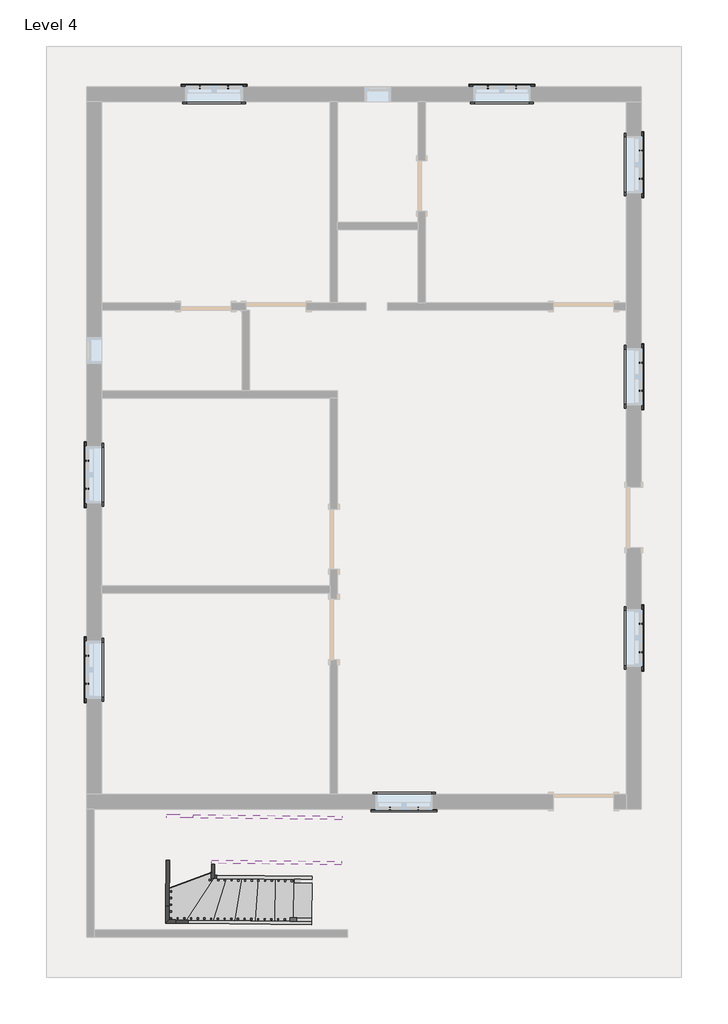
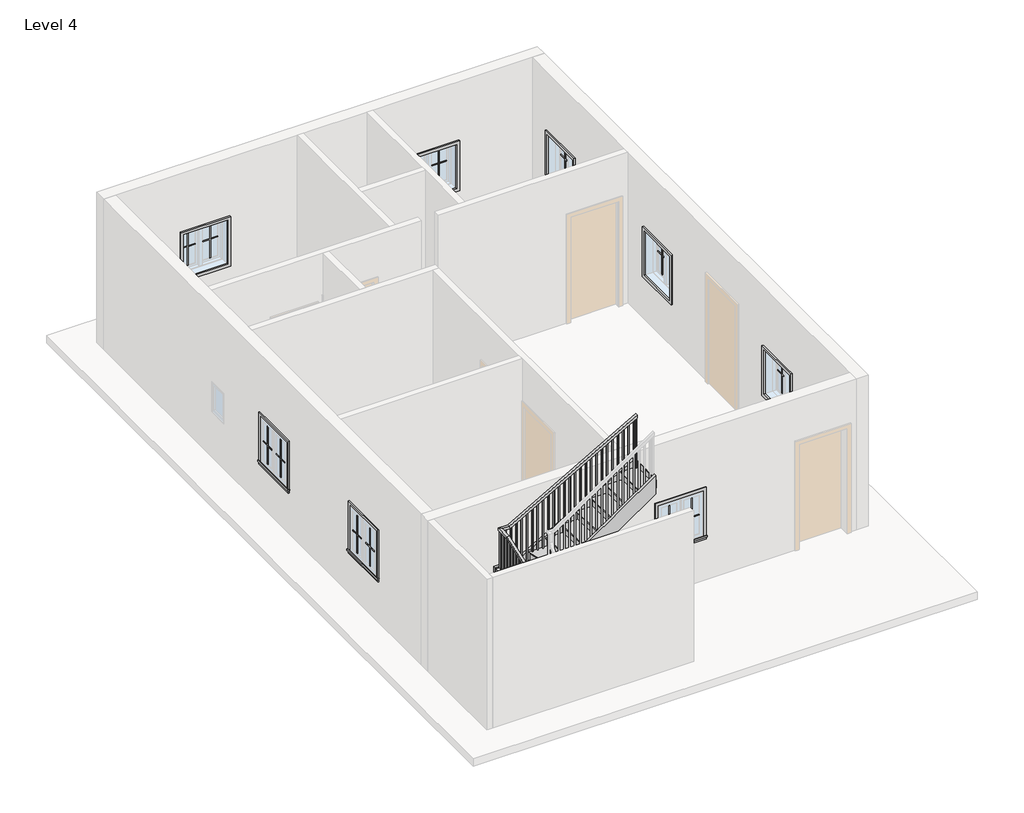
# One storey, part 2 of 2: 32 proxies, 9 members, 1 railing, 1 stair flight.
"""IFC4 building model written with IfcOpenShell, lengths in millimetres."""

from ifc_helpers import new_model, si_unit, frame, origin, place, context, project, spatial, polyline, outline, extrude, faceted_brep, transform, mapped, element, save
from components import muntin_pattern_2x2_muntin_pattern_2x2_b3fe6957, muntin_pattern_2x2_muntin_pattern_2x2_3e0ecaf2, trim_window_exterior_flat_with_sill_41619996, trim_window_interior_flat_picture_frame_51c85655, stair_flight_64b704a5

model = new_model("IFC4")

# Units and contexts
model_context = context("Model", 3, world=origin())
ifc_project = project(units=[si_unit("LENGTHUNIT", "METRE", prefix="MILLI")], contexts=[model_context])

# Site, building, storey
site = spatial("IfcSite", under=ifc_project)
building = spatial("IfcBuilding", under=site)
storey = spatial("IfcBuildingStorey", under=building, Name="Level 4", Elevation=6400.8)

# Proxies
placement = place(None, origin())
muntin_pattern_2x2_muntin_pattern_2x2_shape = muntin_pattern_2x2_muntin_pattern_2x2_b3fe6957(model_context)
element("IfcBuildingElementProxy", 1, Name="Muntin Pattern_2x2 : Muntin Pattern_2x2", ObjectType="Muntin Pattern_2x2 : Muntin Pattern_2x2", at=placement, inside=storey, context=model_context, shape_type="MappedRepresentation", body=[
    mapped(muntin_pattern_2x2_muntin_pattern_2x2_shape, transform((-3662.5622832, 7052.6782079, 7385.05), x_axis=(1.0, 0.0, 0.0), y_axis=(0.0, 1.0, 0.0), z_axis=(0.0, 0.0, 1.0))),
])
element("IfcBuildingElementProxy", 2, Name="Muntin Pattern_2x2 : Muntin Pattern_2x2", ObjectType="Muntin Pattern_2x2 : Muntin Pattern_2x2", at=placement, inside=storey, context=model_context, shape_type="MappedRepresentation", body=[
    mapped(muntin_pattern_2x2_muntin_pattern_2x2_shape, transform((709.4127168, 7052.6782079, 7385.05), x_axis=(1.0, 0.0, 0.0), y_axis=(0.0, 1.0, 0.0), z_axis=(0.0, 0.0, 1.0))),
])
element("IfcBuildingElementProxy", 3, Name="Muntin Pattern_2x2 : Muntin Pattern_2x2", ObjectType="Muntin Pattern_2x2 : Muntin Pattern_2x2", at=placement, inside=storey, context=model_context, shape_type="MappedRepresentation", body=[
    mapped(muntin_pattern_2x2_muntin_pattern_2x2_shape, transform((3028.7502168, 6095.4157079, 7385.05), x_axis=(0.0, -1.0, 0.0), y_axis=(1.0, 0.0, 0.0), z_axis=(0.0, 0.0, 1.0))),
])
element("IfcBuildingElementProxy", 4, Name="Muntin Pattern_2x2 : Muntin Pattern_2x2", ObjectType="Muntin Pattern_2x2 : Muntin Pattern_2x2", at=placement, inside=storey, context=model_context, shape_type="MappedRepresentation", body=[
    mapped(muntin_pattern_2x2_muntin_pattern_2x2_shape, transform((3028.7502168, 2875.9657079, 7385.05), x_axis=(0.0, -1.0, 0.0), y_axis=(1.0, 0.0, 0.0), z_axis=(0.0, 0.0, 1.0))),
])
element("IfcBuildingElementProxy", 5, Name="Muntin Pattern_2x2 : Muntin Pattern_2x2", ObjectType="Muntin Pattern_2x2 : Muntin Pattern_2x2", at=placement, inside=storey, context=model_context, shape_type="MappedRepresentation", body=[
    mapped(muntin_pattern_2x2_muntin_pattern_2x2_shape, transform((3028.7502168, -1086.4342921, 7385.05), x_axis=(0.0, -1.0, 0.0), y_axis=(1.0, 0.0, 0.0), z_axis=(0.0, 0.0, 1.0))),
])
element("IfcBuildingElementProxy", 6, Name="Muntin Pattern_2x2 : Muntin Pattern_2x2", ObjectType="Muntin Pattern_2x2 : Muntin Pattern_2x2", at=placement, inside=storey, context=model_context, shape_type="MappedRepresentation", body=[
    mapped(muntin_pattern_2x2_muntin_pattern_2x2_shape, transform((-5372.2997832, 961.4407079, 7385.05), x_axis=(0.0, 1.0, 0.0), y_axis=(-1.0, 0.0, 0.0), z_axis=(0.0, 0.0, 1.0))),
])
element("IfcBuildingElementProxy", 7, Name="Muntin Pattern_2x2 : Muntin Pattern_2x2", ObjectType="Muntin Pattern_2x2 : Muntin Pattern_2x2", at=placement, inside=storey, context=model_context, shape_type="MappedRepresentation", body=[
    mapped(muntin_pattern_2x2_muntin_pattern_2x2_shape, transform((-5372.2997832, -1997.6592921, 7385.05), x_axis=(0.0, 1.0, 0.0), y_axis=(-1.0, 0.0, 0.0), z_axis=(0.0, 0.0, 1.0))),
])
element("IfcBuildingElementProxy", 8, Name="Muntin Pattern_2x2 : Muntin Pattern_2x2", ObjectType="Muntin Pattern_2x2 : Muntin Pattern_2x2", at=placement, inside=storey, context=model_context, shape_type="MappedRepresentation", body=[
    mapped(muntin_pattern_2x2_muntin_pattern_2x2_shape, transform((-347.8622832, -3888.3717921, 7385.05), x_axis=(-1.0, 0.0, 0.0), y_axis=(0.0, -1.0, 0.0), z_axis=(0.0, 0.0, 1.0))),
])
muntin_pattern_2x2_muntin_pattern_2x2_2_shape = muntin_pattern_2x2_muntin_pattern_2x2_3e0ecaf2(model_context)
element("IfcBuildingElementProxy", 9, Name="Muntin Pattern_2x2 : Muntin Pattern_2x2", ObjectType="Muntin Pattern_2x2 : Muntin Pattern_2x2", at=placement, inside=storey, context=model_context, shape_type="MappedRepresentation", body=[
    mapped(muntin_pattern_2x2_muntin_pattern_2x2_2_shape, transform((-3233.9372832, 7052.6782079, 7385.05), x_axis=(-1.0, 0.0, 0.0), y_axis=(0.0, -1.0, 0.0), z_axis=(0.0, 0.0, 1.0))),
])
element("IfcBuildingElementProxy", 10, Name="Muntin Pattern_2x2 : Muntin Pattern_2x2", ObjectType="Muntin Pattern_2x2 : Muntin Pattern_2x2", at=placement, inside=storey, context=model_context, shape_type="MappedRepresentation", body=[
    mapped(muntin_pattern_2x2_muntin_pattern_2x2_2_shape, transform((1138.0377168, 7052.6782079, 7385.05), x_axis=(-1.0, 0.0, 0.0), y_axis=(0.0, -1.0, 0.0), z_axis=(0.0, 0.0, 1.0))),
])
element("IfcBuildingElementProxy", 11, Name="Muntin Pattern_2x2 : Muntin Pattern_2x2", ObjectType="Muntin Pattern_2x2 : Muntin Pattern_2x2", at=placement, inside=storey, context=model_context, shape_type="MappedRepresentation", body=[
    mapped(muntin_pattern_2x2_muntin_pattern_2x2_2_shape, transform((3028.7502168, 5666.7907079, 7385.05), x_axis=(0.0, 1.0, 0.0), y_axis=(-1.0, 0.0, 0.0), z_axis=(0.0, 0.0, 1.0))),
])
element("IfcBuildingElementProxy", 12, Name="Muntin Pattern_2x2 : Muntin Pattern_2x2", ObjectType="Muntin Pattern_2x2 : Muntin Pattern_2x2", at=placement, inside=storey, context=model_context, shape_type="MappedRepresentation", body=[
    mapped(muntin_pattern_2x2_muntin_pattern_2x2_2_shape, transform((3028.7502168, 2447.3407079, 7385.05), x_axis=(0.0, 1.0, 0.0), y_axis=(-1.0, 0.0, 0.0), z_axis=(0.0, 0.0, 1.0))),
])
element("IfcBuildingElementProxy", 13, Name="Muntin Pattern_2x2 : Muntin Pattern_2x2", ObjectType="Muntin Pattern_2x2 : Muntin Pattern_2x2", at=placement, inside=storey, context=model_context, shape_type="MappedRepresentation", body=[
    mapped(muntin_pattern_2x2_muntin_pattern_2x2_2_shape, transform((3028.7502168, -1515.0592921, 7385.05), x_axis=(0.0, 1.0, 0.0), y_axis=(-1.0, 0.0, 0.0), z_axis=(0.0, 0.0, 1.0))),
])
element("IfcBuildingElementProxy", 14, Name="Muntin Pattern_2x2 : Muntin Pattern_2x2", ObjectType="Muntin Pattern_2x2 : Muntin Pattern_2x2", at=placement, inside=storey, context=model_context, shape_type="MappedRepresentation", body=[
    mapped(muntin_pattern_2x2_muntin_pattern_2x2_2_shape, transform((-5372.2997832, 1390.0657079, 7385.05), x_axis=(0.0, -1.0, 0.0), y_axis=(1.0, 0.0, 0.0), z_axis=(0.0, 0.0, 1.0))),
])
element("IfcBuildingElementProxy", 15, Name="Muntin Pattern_2x2 : Muntin Pattern_2x2", ObjectType="Muntin Pattern_2x2 : Muntin Pattern_2x2", at=placement, inside=storey, context=model_context, shape_type="MappedRepresentation", body=[
    mapped(muntin_pattern_2x2_muntin_pattern_2x2_2_shape, transform((-5372.2997832, -1569.0342921, 7385.05), x_axis=(0.0, -1.0, 0.0), y_axis=(1.0, 0.0, 0.0), z_axis=(0.0, 0.0, 1.0))),
])
element("IfcBuildingElementProxy", 16, Name="Muntin Pattern_2x2 : Muntin Pattern_2x2", ObjectType="Muntin Pattern_2x2 : Muntin Pattern_2x2", at=placement, inside=storey, context=model_context, shape_type="MappedRepresentation", body=[
    mapped(muntin_pattern_2x2_muntin_pattern_2x2_2_shape, transform((-776.4872832, -3888.3717921, 7385.05), x_axis=(1.0, 0.0, 0.0), y_axis=(0.0, 1.0, 0.0), z_axis=(0.0, 0.0, 1.0))),
])
trim_window_exterior_flat_with_sill_shape = trim_window_exterior_flat_with_sill_41619996(model_context)
element("IfcBuildingElementProxy", 17, Name="Trim-Window-Exterior-Flat : with Sill", ObjectType="Trim-Window-Exterior-Flat : with Sill", at=placement, inside=storey, context=model_context, shape_type="MappedRepresentation", body=[
    mapped(trim_window_exterior_flat_with_sill_shape, transform((-3448.2497832, 7062.2032079, 8229.6), x_axis=(-1.0, 0.0, 0.0), y_axis=(0.0, 0.0, 1.0), z_axis=(0.0, 1.0, 0.0))),
])
element("IfcBuildingElementProxy", 18, Name="Trim-Window-Exterior-Flat : with Sill", ObjectType="Trim-Window-Exterior-Flat : with Sill", at=placement, inside=storey, context=model_context, shape_type="MappedRepresentation", body=[
    mapped(trim_window_exterior_flat_with_sill_shape, transform((923.7252168, 7062.2032079, 8229.6), x_axis=(-1.0, 0.0, 0.0), y_axis=(0.0, 0.0, 1.0), z_axis=(0.0, 1.0, 0.0))),
])
element("IfcBuildingElementProxy", 19, Name="Trim-Window-Exterior-Flat : with Sill", ObjectType="Trim-Window-Exterior-Flat : with Sill", at=placement, inside=storey, context=model_context, shape_type="MappedRepresentation", body=[
    mapped(trim_window_exterior_flat_with_sill_shape, transform((3038.2752168, 5881.1032079, 8229.6), x_axis=(0.0, 1.0, 0.0), y_axis=(0.0, 0.0, 1.0), z_axis=(1.0, 0.0, 0.0))),
])
element("IfcBuildingElementProxy", 20, Name="Trim-Window-Exterior-Flat : with Sill", ObjectType="Trim-Window-Exterior-Flat : with Sill", at=placement, inside=storey, context=model_context, shape_type="MappedRepresentation", body=[
    mapped(trim_window_exterior_flat_with_sill_shape, transform((3038.2752168, 2661.6532079, 8229.6), x_axis=(0.0, 1.0, 0.0), y_axis=(0.0, 0.0, 1.0), z_axis=(1.0, 0.0, 0.0))),
])
element("IfcBuildingElementProxy", 21, Name="Trim-Window-Exterior-Flat : with Sill", ObjectType="Trim-Window-Exterior-Flat : with Sill", at=placement, inside=storey, context=model_context, shape_type="MappedRepresentation", body=[
    mapped(trim_window_exterior_flat_with_sill_shape, transform((3038.2752168, -1300.7467921, 8229.6), x_axis=(0.0, 1.0, 0.0), y_axis=(0.0, 0.0, 1.0), z_axis=(1.0, 0.0, 0.0))),
])
element("IfcBuildingElementProxy", 22, Name="Trim-Window-Exterior-Flat : with Sill", ObjectType="Trim-Window-Exterior-Flat : with Sill", at=placement, inside=storey, context=model_context, shape_type="MappedRepresentation", body=[
    mapped(trim_window_exterior_flat_with_sill_shape, transform((-5381.8247832, 1175.7532079, 8229.6), x_axis=(0.0, -1.0, 0.0), y_axis=(0.0, 0.0, 1.0), z_axis=(-1.0, 0.0, 0.0))),
])
element("IfcBuildingElementProxy", 23, Name="Trim-Window-Exterior-Flat : with Sill", ObjectType="Trim-Window-Exterior-Flat : with Sill", at=placement, inside=storey, context=model_context, shape_type="MappedRepresentation", body=[
    mapped(trim_window_exterior_flat_with_sill_shape, transform((-5381.8247832, -1783.3467921, 8229.6), x_axis=(0.0, -1.0, 0.0), y_axis=(0.0, 0.0, 1.0), z_axis=(-1.0, 0.0, 0.0))),
])
element("IfcBuildingElementProxy", 24, Name="Trim-Window-Exterior-Flat : with Sill", ObjectType="Trim-Window-Exterior-Flat : with Sill", at=placement, inside=storey, context=model_context, shape_type="MappedRepresentation", body=[
    mapped(trim_window_exterior_flat_with_sill_shape, transform((-562.1747832, -3897.8967921, 8229.6), x_axis=(1.0, 0.0, 0.0), y_axis=(0.0, 0.0, 1.0), z_axis=(0.0, -1.0, 0.0))),
])
trim_window_interior_flat_picture_frame_shape = trim_window_interior_flat_picture_frame_51c85655(model_context)
element("IfcBuildingElementProxy", 25, Name="Trim-Window-Interior-Flat : Picture Frame", ObjectType="Trim-Window-Interior-Flat : Picture Frame", at=placement, inside=storey, context=model_context, shape_type="MappedRepresentation", body=[
    mapped(trim_window_interior_flat_picture_frame_shape, transform((-3448.2497832, 6833.6032079, 8229.6), x_axis=(1.0, 0.0, 0.0), y_axis=(0.0, 0.0, 1.0), z_axis=(0.0, -1.0, 0.0))),
])
element("IfcBuildingElementProxy", 26, Name="Trim-Window-Interior-Flat : Picture Frame", ObjectType="Trim-Window-Interior-Flat : Picture Frame", at=placement, inside=storey, context=model_context, shape_type="MappedRepresentation", body=[
    mapped(trim_window_interior_flat_picture_frame_shape, transform((923.7252168, 6833.6032079, 8229.6), x_axis=(1.0, 0.0, 0.0), y_axis=(0.0, 0.0, 1.0), z_axis=(0.0, -1.0, 0.0))),
])
element("IfcBuildingElementProxy", 27, Name="Trim-Window-Interior-Flat : Picture Frame", ObjectType="Trim-Window-Interior-Flat : Picture Frame", at=placement, inside=storey, context=model_context, shape_type="MappedRepresentation", body=[
    mapped(trim_window_interior_flat_picture_frame_shape, transform((2809.6752168, 5881.1032079, 8229.6), x_axis=(0.0, -1.0, 0.0), y_axis=(0.0, 0.0, 1.0), z_axis=(-1.0, 0.0, 0.0))),
])
element("IfcBuildingElementProxy", 28, Name="Trim-Window-Interior-Flat : Picture Frame", ObjectType="Trim-Window-Interior-Flat : Picture Frame", at=placement, inside=storey, context=model_context, shape_type="MappedRepresentation", body=[
    mapped(trim_window_interior_flat_picture_frame_shape, transform((2809.6752168, 2661.6532079, 8229.6), x_axis=(0.0, -1.0, 0.0), y_axis=(0.0, 0.0, 1.0), z_axis=(-1.0, 0.0, 0.0))),
])
element("IfcBuildingElementProxy", 29, Name="Trim-Window-Interior-Flat : Picture Frame", ObjectType="Trim-Window-Interior-Flat : Picture Frame", at=placement, inside=storey, context=model_context, shape_type="MappedRepresentation", body=[
    mapped(trim_window_interior_flat_picture_frame_shape, transform((2809.6752168, -1300.7467921, 8229.6), x_axis=(0.0, -1.0, 0.0), y_axis=(0.0, 0.0, 1.0), z_axis=(-1.0, 0.0, 0.0))),
])
element("IfcBuildingElementProxy", 30, Name="Trim-Window-Interior-Flat : Picture Frame", ObjectType="Trim-Window-Interior-Flat : Picture Frame", at=placement, inside=storey, context=model_context, shape_type="MappedRepresentation", body=[
    mapped(trim_window_interior_flat_picture_frame_shape, transform((-5153.2247832, 1175.7532079, 8229.6), x_axis=(0.0, 1.0, 0.0), y_axis=(0.0, 0.0, 1.0), z_axis=(1.0, 0.0, 0.0))),
])
element("IfcBuildingElementProxy", 31, Name="Trim-Window-Interior-Flat : Picture Frame", ObjectType="Trim-Window-Interior-Flat : Picture Frame", at=placement, inside=storey, context=model_context, shape_type="MappedRepresentation", body=[
    mapped(trim_window_interior_flat_picture_frame_shape, transform((-5153.2247832, -1783.3467921, 8229.6), x_axis=(0.0, 1.0, 0.0), y_axis=(0.0, 0.0, 1.0), z_axis=(1.0, 0.0, 0.0))),
])
element("IfcBuildingElementProxy", 32, Name="Trim-Window-Interior-Flat : Picture Frame", ObjectType="Trim-Window-Interior-Flat : Picture Frame", at=placement, inside=storey, context=model_context, shape_type="MappedRepresentation", body=[
    mapped(trim_window_interior_flat_picture_frame_shape, transform((-562.1747832, -3669.2967921, 8229.6), x_axis=(-1.0, 0.0, 0.0), y_axis=(0.0, 0.0, 1.0), z_axis=(0.0, 1.0, 0.0))),
])

# Members
element("IfcMember", 33, ObjectType="Stringer - 2\" Width", at=placement, inside=storey, context=model_context, shape_type="SweptSolid", body=[
    extrude(outline(polyline([(-105.6395382, -202.4353776), (0.0, 0.0), (2328.2458671, 0.0), (2169.1880402, -304.8), (90.52017, -304.8), (-105.6395382, -202.4353776)])), frame((-1968.9977307, -5651.1672049, 6629.1413982), z_axis=(0.010736031619565219, 0.9999423671517594, 0.0), x_axis=(-0.8864958884204132, 0.009517996437940353, 0.46263857119517154)), (0.0, 0.0, 1.0), 50.8),
])
element("IfcMember", 34, ObjectType="Stringer - 2\" Width", at=placement, inside=storey, context=model_context, shape_type="SweptSolid", body=[
    extrude(outline(polyline([(-4032.4327287, -5578.2098967), (-4032.9781191, -5629.006969), (-4182.4018504, -5627.4026586), (-4131.0593878, -5577.1509768), (-4032.4327287, -5578.2098967)])), frame((0.0, 0.0, 7362.4719334), z_axis=(0.0, 0.0, 1.0), x_axis=(1.0, 0.0, 0.0)), (0.0, 0.0, 1.0), 343.8058061),
])
element("IfcMember", 35, ObjectType="Stringer - 2\" Width", at=placement, inside=storey, context=model_context, shape_type="SweptSolid", body=[
    extrude(outline(polyline([(-4131.0593878, -5577.1509768), (-4182.4018504, -5627.4026586), (-4179.6442274, -5370.5606366), (-4128.8471552, -5371.106027), (-4131.0593878, -5577.1509768)])), frame((0.0, 0.0, 7362.4719334), z_axis=(0.0, 0.0, 1.0), x_axis=(1.0, 0.0, 0.0)), (0.0, 0.0, 1.0), 343.8058061),
])
element("IfcMember", 36, ObjectType="Stringer - 2\" Width", at=placement, inside=storey, context=model_context, shape_type="SweptSolid", body=[
    extrude(outline(polyline([(110.9788635, -325.4014815), (0.0, 0.0), (1419.3210826, 0.0), (1526.5904374, -314.5248191), (1494.6989405, -325.4014816), (110.9788635, -325.4014815)])), frame((-4128.8471552, -5371.106027, 7362.4719334), z_axis=(-0.9999423671517593, 0.010736031619565298, 0.0), x_axis=(0.010161319362697869, 0.946414289466532, 0.3227951986668461)), (0.0, 0.0, 1.0), 50.8),
])
element("IfcMember", 37, ObjectType="Stringer - 2\" Width", at=placement, inside=storey, context=model_context, shape_type="SweptSolid", body=[
    extrude(outline(polyline([(-4165.2220526, -4027.2948827), (-4164.6766622, -3976.4978105), (-3763.6581151, -3980.8034064), (-3764.2035055, -4031.6004787), (-4165.2220526, -4027.2948827)])), frame((0.0, 0.0, 7830.8968076), z_axis=(0.0, 0.0, 1.0), x_axis=(1.0, 0.0, 0.0)), (0.0, 0.0, 1.0), 322.0391291),
])
element("IfcMember", 38, ObjectType="Stringer - 2\" Width", at=placement, inside=storey, context=model_context, shape_type="SweptSolid", body=[
    extrude(outline(polyline([(-111.9640108, -160.4153284), (0.0, 0.0), (1801.1015507, 0.0), (1588.362339, -304.8), (94.9016984, -304.8), (-111.9640108, -160.4153284)])), frame((-1961.6349602, -4965.4067295, 6596.4246848), z_axis=(0.010736031619565368, 0.9999423671517594, 0.0), x_axis=(-0.819968519558025, 0.008803715336213085, 0.5723409137307064)), (0.0, 0.0, 1.0), 50.8),
])
element("IfcMember", 39, ObjectType="Stringer - 2\" Width", at=placement, inside=storey, context=model_context, shape_type="SweptSolid", body=[
    extrude(outline(polyline([(451.3522078, -304.8), (7.554265, -5.1014262), (10.999279, 0.0), (408.4725128, 0.0), (831.8908901, -285.9361695), (819.1520678, -304.8), (451.3522078, -304.8)])), frame((-3438.4815323, -4949.5503441, 7281.9097108), z_axis=(-0.9999423671517593, 0.010736031619565902, 0.0), x_axis=(0.006008376943933788, 0.559613726649971, 0.8287317879455518)), (0.0, 0.0, 1.0), 50.8),
])
element("IfcMember", 40, ObjectType="Stringer - 2\" Width", at=placement, inside=storey, context=model_context, shape_type="SweptSolid", body=[
    extrude(outline(polyline([(215.732707, -304.8), (0.0, 0.0), (2421.4097535, 0.0), (2637.1424605, -304.8), (215.732707, -304.8)])), frame((-3486.8243477, -4720.4181286, 7757.9256311), z_axis=(0.010736031619565212, 0.9999423671517594, 0.0), x_axis=(0.8161886957592969, -0.008763132689499908, 0.5777189804915571)), (0.0, 0.0, 1.0), 50.8),
])
element("IfcMember", 41, ObjectType="Stringer - 2\" Width", at=placement, inside=storey, context=model_context, shape_type="SweptSolid", body=[
    extrude(outline(polyline([(161.6856691, -278.5084291), (0.0, 0.0), (2614.6236412, 0.0), (2776.3093103, -278.508429), (161.6856691, -278.5084291)])), frame((-3764.2035055, -4031.6004787, 7830.8968076), z_axis=(0.010736031619565317, 0.9999423671517593, 0.0), x_axis=(0.8647780740833303, -0.009284819857879245, 0.5020683964410952)), (0.0, 0.0, 1.0), 50.8),
])

# Railing
element("IfcRailing", 42, ObjectType="Handrail - Rectangular", at=placement, inside=storey, context=model_context, shape_type="SolidModel", body=[
    faceted_brep([(-1968.4523403, -5600.3701326, 7484.5333333), (-1968.4523403, -5600.3701326, 7426.9388957), (-1967.9069499, -5549.5730604, 7426.9388957), (-1967.9069499, -5549.5730604, 7484.5333333), (-4009.5042766, -5578.4560715, 8574.9579081), (-4022.2220752, -5578.319525, 8524.1579081), (-4021.6766848, -5527.5224527, 8524.1579081), (-4008.9588862, -5527.6589993, 8574.9579081), (-4131.0593878, -5577.1509768, 8574.9579081), (-4131.0593878, -5577.1509768, 8524.1579081), (-4079.7169251, -5526.8992949, 8524.1579081), (-4079.7169251, -5526.8992949, 8574.9579081), (-4129.1695675, -5401.1351667, 8574.9579081), (-4129.079122, -5392.7111679, 8524.1579081), (-4078.2820498, -5393.2565584, 8524.1579081), (-4078.3724953, -5401.6805571, 8574.9579081), (-4117.5603361, -4319.8639155, 8943.7490097), (-4117.4698906, -4311.4399167, 8892.9490097), (-4066.6728183, -4311.9853071, 8892.9490097), (-4066.7632639, -4320.4093059, 8943.7490097), (-4114.4249804, -4027.8402731, 8943.7490097), (-4114.4249804, -4027.8402731, 8892.9490097), (-4064.1732985, -4079.1827358, 8892.9490097), (-4064.1732985, -4079.1827358, 8943.7490097), (-3933.3337165, -4029.7845867, 8943.7490097), (-3919.5861077, -4029.93219, 8892.9490097), (-3920.1314981, -4080.7292622, 8892.9490097), (-3933.8791069, -4080.581659, 8943.7490097), (-1503.1343086, -4055.8767882, 10363.2), (-1503.679699, -4106.6738604, 10363.2), (-1503.679699, -4106.6738604, 10304.3701828), (-1503.1343086, -4055.8767882, 10304.3701828)], [[[0, 1, 2, 3]], [[1, 0, 4, 5]], [[2, 1, 5, 6]], [[3, 2, 6, 7]], [[0, 3, 7, 4]], [[5, 4, 8, 9]], [[6, 5, 9, 10]], [[7, 6, 10, 11]], [[4, 7, 11, 8]], [[9, 8, 12, 13]], [[10, 9, 13, 14]], [[11, 10, 14, 15]], [[8, 11, 15, 12]], [[13, 12, 16, 17]], [[14, 13, 17, 18]], [[15, 14, 18, 19]], [[12, 15, 19, 16]], [[17, 16, 20, 21]], [[18, 17, 21, 22]], [[19, 18, 22, 23]], [[16, 19, 23, 20]], [[21, 20, 24, 25]], [[22, 21, 25, 26]], [[23, 22, 26, 27]], [[20, 23, 27, 24]], [[28, 29, 30, 31]], [[25, 24, 28, 31]], [[26, 25, 31, 30]], [[27, 26, 30, 29]], [[24, 27, 29, 28]]]),
    extrude(outline(polyline([(234.1631202, 19.05), (1226.6129544, 19.05), (1226.6129544, 0.0), (223.0368797, 0.0), (234.1631202, 19.05)])), frame((-1540.0233365, -4090.4077365, 10506.0796211), z_axis=(0.010736031619565153, 0.9999423671517594, 0.0), x_axis=(0.0, 0.0, -1.0)), (0.0, 0.0, 1.0), 19.05),
    extrude(outline(polyline([(234.1631202, 19.05), (1167.2730054, 19.05), (1167.2730054, 0.0), (223.0368798, 0.0), (234.1631202, 19.05)])), frame((-1641.617481, -4089.3169557, 10446.7396721), z_axis=(0.010736031619565153, 0.9999423671517594, 0.0), x_axis=(0.0, 0.0, -1.0)), (0.0, 0.0, 1.0), 19.05),
    extrude(outline(polyline([(234.1631202, 19.05), (1107.9330563, 19.05), (1107.9330563, 0.0), (223.0368797, 0.0), (234.1631202, 19.05)])), frame((-1743.2116255, -4088.2261749, 10387.399723), z_axis=(0.010736031619565153, 0.9999423671517594, 0.0), x_axis=(0.0, 0.0, -1.0)), (0.0, 0.0, 1.0), 19.05),
    extrude(outline(polyline([(234.1631202, 19.05), (1217.9264407, 19.05), (1217.9264407, 0.0), (223.0368798, 0.0), (234.1631202, 19.05)])), frame((-1844.80577, -4087.1353941, 10328.059774), z_axis=(0.010736031619565153, 0.9999423671517594, 0.0), x_axis=(0.0, 0.0, -1.0)), (0.0, 0.0, 1.0), 19.05),
    extrude(outline(polyline([(234.1631203, 19.05), (1158.5864917, 19.05), (1158.5864917, 0.0), (223.0368798, 0.0), (234.1631203, 19.05)])), frame((-1946.3999145, -4086.0446133, 10268.719825), z_axis=(0.010736031619565153, 0.9999423671517594, 0.0), x_axis=(0.0, 0.0, -1.0)), (0.0, 0.0, 1.0), 19.05),
    extrude(outline(polyline([(234.1631202, 19.05), (1099.2465426, 19.05), (1099.2465426, 0.0), (223.0368798, 0.0), (234.1631202, 19.05)])), frame((-2047.994059, -4084.9538324, 10209.3798759), z_axis=(0.010736031619565153, 0.9999423671517594, 0.0), x_axis=(0.0, 0.0, -1.0)), (0.0, 0.0, 1.0), 19.05),
    extrude(outline(polyline([(234.1631202, 19.0499999), (1209.2399269, 19.0499999), (1209.2399269, 0.0), (223.0368798, 0.0), (234.1631202, 19.0499999)])), frame((-2149.5882036, -4083.8630516, 10150.0399269), z_axis=(0.010736031619565153, 0.9999423671517594, 0.0), x_axis=(0.0, 0.0, -1.0)), (0.0, 0.0, 1.0), 19.05),
    extrude(outline(polyline([(234.1631202, 19.0499999), (1149.8999778, 19.0499999), (1149.8999778, 0.0), (223.0368797, 0.0), (234.1631202, 19.0499999)])), frame((-2251.1823481, -4082.7722708, 10090.6999778), z_axis=(0.010736031619565153, 0.9999423671517594, 0.0), x_axis=(0.0, 0.0, -1.0)), (0.0, 0.0, 1.0), 19.05),
    extrude(outline(polyline([(234.1631202, 19.05), (1259.8933621, 19.05), (1259.8933621, 0.0), (223.0368798, 0.0), (234.1631202, 19.05)])), frame((-2352.7764926, -4081.68149, 10031.3600288), z_axis=(0.010736031619565153, 0.9999423671517594, 0.0), x_axis=(0.0, 0.0, -1.0)), (0.0, 0.0, 1.0), 19.05),
    extrude(outline(polyline([(234.1631203, 19.05), (1200.5534131, 19.05), (1200.5534131, 0.0), (223.0368798, 0.0), (234.1631203, 19.05)])), frame((-2454.3706371, -4080.5907092, 9972.0200798), z_axis=(0.010736031619565153, 0.9999423671517594, 0.0), x_axis=(0.0, 0.0, -1.0)), (0.0, 0.0, 1.0), 19.05),
    extrude(outline(polyline([(234.1631202, 19.05), (1141.213464, 19.05), (1141.213464, 0.0), (223.0368798, 0.0), (234.1631202, 19.05)])), frame((-2555.9647816, -4079.4999284, 9912.6801307), z_axis=(0.010736031619565153, 0.9999423671517594, 0.0), x_axis=(0.0, 0.0, -1.0)), (0.0, 0.0, 1.0), 19.05),
    extrude(outline(polyline([(234.1631203, 19.05), (1251.2068484, 19.05), (1251.2068484, 0.0), (223.0368798, 0.0), (234.1631203, 19.05)])), frame((-2657.5589261, -4078.4091476, 9853.3401817), z_axis=(0.010736031619565153, 0.9999423671517594, 0.0), x_axis=(0.0, 0.0, -1.0)), (0.0, 0.0, 1.0), 19.05),
    extrude(outline(polyline([(234.1631202, 19.05), (1191.8668993, 19.05), (1191.8668993, 0.0), (223.0368797, 0.0), (234.1631202, 19.05)])), frame((-2759.1530706, -4077.3183668, 9794.0002326), z_axis=(0.010736031619565153, 0.9999423671517594, 0.0), x_axis=(0.0, 0.0, -1.0)), (0.0, 0.0, 1.0), 19.05),
    extrude(outline(polyline([(234.1631202, 19.05), (1132.5269503, 19.05), (1132.5269503, 0.0), (223.0368798, 0.0), (234.1631202, 19.05)])), frame((-2860.7472151, -4076.2275859, 9734.6602836), z_axis=(0.010736031619565153, 0.9999423671517594, 0.0), x_axis=(0.0, 0.0, -1.0)), (0.0, 0.0, 1.0), 19.05),
    extrude(outline(polyline([(234.1631202, 19.05), (1242.5203345, 19.05), (1242.5203345, 0.0), (223.0368797, 0.0), (234.1631202, 19.05)])), frame((-2962.3413596, -4075.1368051, 9675.3203345), z_axis=(0.010736031619565153, 0.9999423671517594, 0.0), x_axis=(0.0, 0.0, -1.0)), (0.0, 0.0, 1.0), 19.05),
    extrude(outline(polyline([(234.1631202, 19.05), (1183.1803855, 19.05), (1183.1803855, 0.0), (223.0368798, 0.0), (234.1631202, 19.05)])), frame((-3063.9355041, -4074.0460243, 9615.9803855), z_axis=(0.010736031619565153, 0.9999423671517594, 0.0), x_axis=(0.0, 0.0, -1.0)), (0.0, 0.0, 1.0), 19.05),
    extrude(outline(polyline([(234.1631203, 19.05), (1123.8404365, 19.05), (1123.8404365, 0.0), (223.0368798, 0.0), (234.1631203, 19.05)])), frame((-3165.5296486, -4072.9552435, 9556.6404365), z_axis=(0.010736031619565153, 0.9999423671517594, 0.0), x_axis=(0.0, 0.0, -1.0)), (0.0, 0.0, 1.0), 19.05),
    extrude(outline(polyline([(234.1631202, 19.05), (1233.8338207, 19.05), (1233.8338207, 0.0), (223.0368798, 0.0), (234.1631202, 19.05)])), frame((-3267.1237931, -4071.8644627, 9497.3004874), z_axis=(0.010736031619565153, 0.9999423671517594, 0.0), x_axis=(0.0, 0.0, -1.0)), (0.0, 0.0, 1.0), 19.05),
    extrude(outline(polyline([(234.1631202, 19.05), (1174.4938717, 19.05), (1174.4938717, 0.0), (223.0368798, 0.0), (234.1631202, 19.05)])), frame((-3368.7179376, -4070.7736819, 9437.9605384), z_axis=(0.010736031619565153, 0.9999423671517594, 0.0), x_axis=(0.0, 0.0, -1.0)), (0.0, 0.0, 1.0), 19.05),
    extrude(outline(polyline([(234.1631202, 19.05), (1115.1539226, 19.05), (1115.1539226, 0.0), (223.0368797, 0.0), (234.1631202, 19.05)])), frame((-3470.3120821, -4069.6829011, 9378.6205893), z_axis=(0.010736031619565153, 0.9999423671517594, 0.0), x_axis=(0.0, 0.0, -1.0)), (0.0, 0.0, 1.0), 19.05),
    extrude(outline(polyline([(234.1631202, 19.05), (1225.147307, 19.05), (1225.147307, 0.0), (223.0368798, 0.0), (234.1631202, 19.05)])), frame((-3571.9062266, -4068.5921203, 9319.2806403), z_axis=(0.010736031619565153, 0.9999423671517594, 0.0), x_axis=(0.0, 0.0, -1.0)), (0.0, 0.0, 1.0), 19.05),
    extrude(outline(polyline([(234.1631202, 19.05), (1165.8073579, 19.05), (1165.8073579, 0.0), (223.0368797, 0.0), (234.1631202, 19.05)])), frame((-3673.5003711, -4067.5013394, 9259.9406912), z_axis=(0.010736031619565153, 0.9999423671517594, 0.0), x_axis=(0.0, 0.0, -1.0)), (0.0, 0.0, 1.0), 19.05),
    extrude(outline(polyline([(234.1631202, 19.05), (1106.4674089, 19.05), (1106.4674089, 0.0), (223.0368798, 0.0), (234.1631202, 19.05)])), frame((-3775.0945156, -4066.4105586, 9200.6007422), z_axis=(0.010736031619565153, 0.9999423671517594, 0.0), x_axis=(0.0, 0.0, -1.0)), (0.0, 0.0, 1.0), 19.05),
    extrude(outline(polyline([(234.1631203, 19.05), (1047.1274599, 19.05), (1047.1274599, 0.0), (223.0368798, 0.0), (234.1631203, 19.05)])), frame((-3876.6886601, -4065.3197778, 9141.2607932), z_axis=(0.010736031619565153, 0.9999423671517594, 0.0), x_axis=(0.0, 0.0, -1.0)), (0.0, 0.0, 1.0), 19.05),
    extrude(outline(polyline([(-3997.1271853, -4044.9755735), (-3978.0782832, -4045.1800949), (-3978.2828046, -4064.228997), (-3997.3317067, -4064.0244756), (-3997.1271853, -4044.9755735)])), frame((0.0, 0.0, 8094.1333333), z_axis=(0.0, 0.0, 1.0), x_axis=(1.0, 0.0, 0.0)), (0.0, 0.0, 1.0), 798.8156763),
    extrude(outline(polyline([(-4099.7439368, -4139.1293032), (-4099.5394154, -4120.0804011), (-4080.4905133, -4120.2849225), (-4080.6950347, -4139.3338246), (-4099.7439368, -4139.1293032)])), frame((0.0, 0.0, 8094.1333333), z_axis=(0.0, 0.0, 1.0), x_axis=(1.0, 0.0, 0.0)), (0.0, 0.0, 1.0), 798.8156763),
    extrude(outline(polyline([(-4100.8347176, -4240.7234477), (-4100.6301962, -4221.6745456), (-4081.5812941, -4221.879067), (-4081.7858155, -4240.9279691), (-4100.8347176, -4240.7234477)])), frame((0.0, 0.0, 7924.8), z_axis=(0.0, 0.0, 1.0), x_axis=(1.0, 0.0, 0.0)), (0.0, 0.0, 1.0), 968.1490097),
    extrude(outline(polyline([(231.8485214, 19.05), (1189.524158, 19.05), (1189.524158, 0.0), (225.3514786, 0.0), (231.8485214, 19.05)])), frame((-4082.6720749, -4323.4732115, 9114.324158), z_axis=(-0.9999423671517593, 0.010736031619565137, 0.0), x_axis=(0.0, 0.0, -1.0)), (0.0, 0.0, 1.0), 19.05),
    extrude(outline(polyline([(231.8485214, 19.05), (1154.8732631, 19.05), (1154.8732631, 0.0), (225.3514786, 0.0), (231.8485214, 19.05)])), frame((-4083.7628557, -4425.067356, 9079.6732631), z_axis=(-0.9999423671517593, 0.010736031619565137, 0.0), x_axis=(0.0, 0.0, -1.0)), (0.0, 0.0, 1.0), 19.05),
    extrude(outline(polyline([(231.8485214, 19.05), (1120.2223682, 19.05), (1120.2223682, 0.0), (225.3514786, 0.0), (231.8485214, 19.05)])), frame((-4084.8536366, -4526.6615005, 9045.0223682), z_axis=(-0.9999423671517593, 0.010736031619565137, 0.0), x_axis=(0.0, 0.0, -1.0)), (0.0, 0.0, 1.0), 19.05),
    extrude(outline(polyline([(231.8485214, 19.05), (1085.5714733, 19.05), (1085.5714733, 0.0), (225.3514786, 0.0), (231.8485214, 19.05)])), frame((-4085.9444174, -4628.255645, 9010.3714733), z_axis=(-0.9999423671517593, 0.010736031619565137, 0.0), x_axis=(0.0, 0.0, -1.0)), (0.0, 0.0, 1.0), 19.05),
    extrude(outline(polyline([(231.8485214, 19.05), (1220.2539118, 19.05), (1220.2539118, 0.0), (225.3514786, 0.0), (231.8485214, 19.05)])), frame((-4087.0351982, -4729.8497895, 8975.7205785), z_axis=(-0.9999423671517593, 0.010736031619565137, 0.0), x_axis=(0.0, 0.0, -1.0)), (0.0, 0.0, 1.0), 19.05),
    extrude(outline(polyline([(231.8485214, 19.05), (1185.6030169, 19.05), (1185.6030169, 0.0), (225.3514786, 0.0), (231.8485214, 19.05)])), frame((-4088.125979, -4831.443934, 8941.0696836), z_axis=(-0.9999423671517593, 0.010736031619565137, 0.0), x_axis=(0.0, 0.0, -1.0)), (0.0, 0.0, 1.0), 19.05),
    extrude(outline(polyline([(231.8485214, 19.05), (1150.952122, 19.05), (1150.952122, 0.0), (225.3514786, 0.0), (231.8485214, 19.05)])), frame((-4089.2167598, -4933.0380785, 8906.4187887), z_axis=(-0.9999423671517593, 0.010736031619565137, 0.0), x_axis=(0.0, 0.0, -1.0)), (0.0, 0.0, 1.0), 19.05),
    extrude(outline(polyline([(231.8485214, 19.05), (1116.3012271, 19.05), (1116.3012271, 0.0), (225.3514786, 0.0), (231.8485214, 19.05)])), frame((-4090.3075406, -5034.632223, 8871.7678938), z_axis=(-0.9999423671517593, 0.010736031619565137, 0.0), x_axis=(0.0, 0.0, -1.0)), (0.0, 0.0, 1.0), 19.05),
    extrude(outline(polyline([(231.8485214, 19.05), (1250.9836656, 19.05), (1250.9836656, 0.0), (225.3514786, 0.0), (231.8485214, 19.05)])), frame((-4091.3983214, -5136.2263675, 8837.1169989), z_axis=(-0.9999423671517593, 0.010736031619565137, 0.0), x_axis=(0.0, 0.0, -1.0)), (0.0, 0.0, 1.0), 19.05),
    extrude(outline(polyline([(231.8485214, 19.05), (1216.3327708, 19.05), (1216.3327708, 0.0), (225.3514786, 0.0), (231.8485214, 19.05)])), frame((-4092.4891022, -5237.820512, 8802.4661041), z_axis=(-0.9999423671517593, 0.010736031619565137, 0.0), x_axis=(0.0, 0.0, -1.0)), (0.0, 0.0, 1.0), 19.05),
    extrude(outline(polyline([(231.8485214, 19.05), (1181.6818759, 19.05), (1181.6818759, 0.0), (225.3514786, 0.0), (231.8485214, 19.05)])), frame((-4093.5798831, -5339.4146565, 8767.8152092), z_axis=(-0.9999423671517593, 0.010736031619565137, 0.0), x_axis=(0.0, 0.0, -1.0)), (0.0, 0.0, 1.0), 19.05),
    extrude(outline(polyline([(-4113.9240874, -5459.8531817), (-4113.719566, -5440.8042796), (-4094.6706639, -5441.008801), (-4094.8751853, -5460.0577031), (-4113.9240874, -5459.8531817)])), frame((0.0, 0.0, 7586.1333333), z_axis=(0.0, 0.0, 1.0), x_axis=(1.0, 0.0, 0.0)), (0.0, 0.0, 1.0), 938.0245748),
    extrude(outline(polyline([(-4092.2344893, -5561.6919112), (-4111.2833914, -5561.4873898), (-4111.07887, -5542.4384877), (-4092.0299679, -5542.6430091), (-4092.2344893, -5561.6919112)])), frame((0.0, 0.0, 7586.1333333), z_axis=(0.0, 0.0, 1.0), x_axis=(1.0, 0.0, 0.0)), (0.0, 0.0, 1.0), 938.0245748),
    extrude(outline(polyline([(223.5115966, 19.05), (1154.9316075, 19.05), (1154.9316075, 0.0), (233.6884033, 0.0), (223.5115966, 19.05)])), frame((-3990.6403448, -5562.782692, 8741.0649408), z_axis=(0.010736031619565252, 0.9999423671517594, 0.0), x_axis=(0.0, 0.0, -1.0)), (0.0, 0.0, 1.0), 19.05),
    extrude(outline(polyline([(223.5115967, 19.05), (1100.6553053, 19.05), (1100.6553053, 0.0), (233.6884034, 0.0), (223.5115967, 19.05)])), frame((-3889.0462003, -5563.8734728, 8686.7886386), z_axis=(0.010736031619565252, 0.9999423671517594, 0.0), x_axis=(0.0, 0.0, -1.0)), (0.0, 0.0, 1.0), 19.05),
    extrude(outline(polyline([(223.5115967, 19.05), (1215.7123363, 19.05), (1215.7123363, 0.0), (233.6884033, 0.0), (223.5115967, 19.05)])), frame((-3787.4520558, -5564.9642536, 8632.5123363), z_axis=(0.010736031619565252, 0.9999423671517594, 0.0), x_axis=(0.0, 0.0, -1.0)), (0.0, 0.0, 1.0), 19.05),
    extrude(outline(polyline([(223.5115967, 19.05), (1161.4360341, 19.05), (1161.4360341, 0.0), (233.6884034, 0.0), (223.5115967, 19.05)])), frame((-3685.8579113, -5566.0550344, 8578.2360341), z_axis=(0.010736031619565252, 0.9999423671517594, 0.0), x_axis=(0.0, 0.0, -1.0)), (0.0, 0.0, 1.0), 19.05),
    extrude(outline(polyline([(223.5115967, 19.05), (1107.1597318, 19.05), (1107.1597318, 0.0), (233.6884033, 0.0), (223.5115967, 19.05)])), frame((-3584.2637668, -5567.1458152, 8523.9597318), z_axis=(0.010736031619565252, 0.9999423671517594, 0.0), x_axis=(0.0, 0.0, -1.0)), (0.0, 0.0, 1.0), 19.05),
    extrude(outline(polyline([(223.5115966, 19.05), (1052.8834295, 19.05), (1052.8834295, 0.0), (233.6884033, 0.0), (223.5115966, 19.05)])), frame((-3482.6696223, -5568.236596, 8469.6834295), z_axis=(0.010736031619565252, 0.9999423671517594, 0.0), x_axis=(0.0, 0.0, -1.0)), (0.0, 0.0, 1.0), 19.05),
    extrude(outline(polyline([(223.5115967, 19.05), (1167.9404606, 19.05), (1167.9404606, 0.0), (233.6884034, 0.0), (223.5115967, 19.05)])), frame((-3381.0754778, -5569.3273769, 8415.4071273), z_axis=(0.010736031619565252, 0.9999423671517594, 0.0), x_axis=(0.0, 0.0, -1.0)), (0.0, 0.0, 1.0), 19.05),
    extrude(outline(polyline([(223.5115966, 19.05), (1113.6641583, 19.05), (1113.6641583, 0.0), (233.6884033, 0.0), (223.5115966, 19.05)])), frame((-3279.4813333, -5570.4181577, 8361.130825), z_axis=(0.010736031619565252, 0.9999423671517594, 0.0), x_axis=(0.0, 0.0, -1.0)), (0.0, 0.0, 1.0), 19.05),
    extrude(outline(polyline([(223.5115967, 19.05), (1059.3878561, 19.05), (1059.3878561, 0.0), (233.6884034, 0.0), (223.5115967, 19.05)])), frame((-3177.8871888, -5571.5089385, 8306.8545228), z_axis=(0.010736031619565252, 0.9999423671517594, 0.0), x_axis=(0.0, 0.0, -1.0)), (0.0, 0.0, 1.0), 19.05),
    extrude(outline(polyline([(223.5115966, 19.05), (1174.4448872, 19.05), (1174.4448872, 0.0), (233.6884033, 0.0), (223.5115966, 19.05)])), frame((-3076.2930443, -5572.5997193, 8252.5782205), z_axis=(0.010736031619565252, 0.9999423671517594, 0.0), x_axis=(0.0, 0.0, -1.0)), (0.0, 0.0, 1.0), 19.05),
    extrude(outline(polyline([(223.5115967, 19.05), (1120.168585, 19.05), (1120.168585, 0.0), (233.6884034, 0.0), (223.5115967, 19.05)])), frame((-2974.6988998, -5573.6905001, 8198.3019183), z_axis=(0.010736031619565252, 0.9999423671517594, 0.0), x_axis=(0.0, 0.0, -1.0)), (0.0, 0.0, 1.0), 19.05),
    extrude(outline(polyline([(223.5115967, 19.05), (1065.8922827, 19.05), (1065.8922827, 0.0), (233.6884033, 0.0), (223.5115967, 19.05)])), frame((-2873.1047553, -5574.7812809, 8144.025616), z_axis=(0.010736031619565252, 0.9999423671517594, 0.0), x_axis=(0.0, 0.0, -1.0)), (0.0, 0.0, 1.0), 19.05),
    extrude(outline(polyline([(223.5115966, 19.05), (1180.9493137, 19.05), (1180.9493137, 0.0), (233.6884033, 0.0), (223.5115966, 19.05)])), frame((-2771.5106108, -5575.8720617, 8089.7493137), z_axis=(0.010736031619565252, 0.9999423671517594, 0.0), x_axis=(0.0, 0.0, -1.0)), (0.0, 0.0, 1.0), 19.05),
    extrude(outline(polyline([(223.5115967, 19.05), (1126.6730115, 19.05), (1126.6730115, 0.0), (233.6884033, 0.0), (223.5115967, 19.05)])), frame((-2669.9164663, -5576.9628425, 8035.4730115), z_axis=(0.010736031619565252, 0.9999423671517594, 0.0), x_axis=(0.0, 0.0, -1.0)), (0.0, 0.0, 1.0), 19.05),
    extrude(outline(polyline([(223.5115966, 19.0499999), (1072.3967092, 19.0499999), (1072.3967092, 0.0), (233.6884033, 0.0), (223.5115966, 19.0499999)])), frame((-2568.3223218, -5578.0536234, 7981.1967092), z_axis=(0.010736031619565252, 0.9999423671517594, 0.0), x_axis=(0.0, 0.0, -1.0)), (0.0, 0.0, 1.0), 19.05),
    extrude(outline(polyline([(223.5115967, 19.0499999), (1187.4537403, 19.0499999), (1187.4537403, 0.0), (233.6884034, 0.0), (223.5115967, 19.0499999)])), frame((-2466.7281773, -5579.1444042, 7926.920407), z_axis=(0.010736031619565252, 0.9999423671517594, 0.0), x_axis=(0.0, 0.0, -1.0)), (0.0, 0.0, 1.0), 19.05),
    extrude(outline(polyline([(223.5115966, 19.05), (1133.177438, 19.05), (1133.177438, 0.0), (233.6884033, 0.0), (223.5115966, 19.05)])), frame((-2365.1340327, -5580.235185, 7872.6441047), z_axis=(0.010736031619565252, 0.9999423671517594, 0.0), x_axis=(0.0, 0.0, -1.0)), (0.0, 0.0, 1.0), 19.05),
    extrude(outline(polyline([(223.5115967, 19.05), (1078.9011358, 19.05), (1078.9011358, 0.0), (233.6884034, 0.0), (223.5115967, 19.05)])), frame((-2263.5398882, -5581.3259658, 7818.3678025), z_axis=(0.010736031619565252, 0.9999423671517594, 0.0), x_axis=(0.0, 0.0, -1.0)), (0.0, 0.0, 1.0), 19.05),
    extrude(outline(polyline([(223.5115967, 19.05), (1193.9581669, 19.05), (1193.9581669, 0.0), (233.6884033, 0.0), (223.5115967, 19.05)])), frame((-2161.9457437, -5582.4167466, 7764.0915002), z_axis=(0.010736031619565252, 0.9999423671517594, 0.0), x_axis=(0.0, 0.0, -1.0)), (0.0, 0.0, 1.0), 19.05),
    extrude(outline(polyline([(223.5115967, 19.05), (1139.6818647, 19.05), (1139.6818647, 0.0), (233.6884034, 0.0), (223.5115967, 19.05)])), frame((-2060.3515992, -5583.5075274, 7709.815198), z_axis=(0.010736031619565252, 0.9999423671517594, 0.0), x_axis=(0.0, 0.0, -1.0)), (0.0, 0.0, 1.0), 19.05),
    extrude(outline(polyline([(-4098.9258512, -4062.9336948), (-4098.7213298, -4043.8847927), (-4079.6724277, -4044.0893141), (-4079.8769491, -4063.1382162), (-4098.9258512, -4062.9336948)])), frame((0.0, 0.0, 8094.1333333), z_axis=(0.0, 0.0, 1.0), x_axis=(1.0, 0.0, 0.0)), (0.0, 0.0, 1.0), 798.8156763),
    extrude(outline(polyline([(-4095.9659661, -5561.6518476), (-4115.0148682, -5561.4473262), (-4114.8103468, -5542.3984241), (-4095.7614447, -5542.6029455), (-4095.9659661, -5561.6518476)])), frame((0.0, 0.0, 7586.1333333), z_axis=(0.0, 0.0, 1.0), x_axis=(1.0, 0.0, 0.0)), (0.0, 0.0, 1.0), 938.0245748),
    extrude(outline(polyline([(234.1631202, 19.05), (1247.9403959, 19.05), (1247.9403959, 0.0), (223.0368798, 0.0), (234.1631202, 19.05)])), frame((-1503.5092645, -4090.7997753, 10527.4070626), z_axis=(0.010736031619565153, 0.9999423671517594, 0.0), x_axis=(0.0, 0.0, -1.0)), (0.0, 0.0, 1.0), 19.05),
    extrude(outline(polyline([(223.5115966, 19.05), (1090.4939657, 19.05), (1090.4939657, 0.0), (233.6884033, 0.0), (223.5115966, 19.05)])), frame((-1968.2819058, -5584.4960475, 7660.627299), z_axis=(0.010736031619565252, 0.9999423671517594, 0.0), x_axis=(0.0, 0.0, -1.0)), (0.0, 0.0, 1.0), 19.05),
])

# Stair flight
stair_flight_shape = stair_flight_64b704a5(model_context)
element("IfcStairFlight", 43, ObjectType="2\" Tread 1\" Nosing 1/4\" Riser", at=placement, inside=storey, context=model_context, shape_type="MappedRepresentation", body=[
    mapped(stair_flight_shape, transform((0.0, 0.0, 0.0), x_axis=(1.0, 0.0, 0.0), y_axis=(0.0, 1.0, 0.0), z_axis=(0.0, 0.0, 1.0))),
])

save(model, "model.ifc")

# Revit data of these elements
# Type "Muntin Pattern_2x2 : Muntin Pattern_2x2"
#   Width [instance default] = 4' - 0"
#   Thickness = 0' - 0 1/2"
#   Height [instance default] = 4' - 0"
#   Distance = 0' - 0 3/4"
#   Interior Material [instance default] = none
#   Exterior Material [instance default] = none
#   Default Elevation = 0
# Type "Trim-Window-Exterior-Flat : with Sill"
#   Trim Width = 0' - 2 1/4"
#   Trim Thickness_Picture Frame = 0' - 1 1/4"
#   Trim Thickness_with Sill = 0' - 0 3/4"
#   Sill Thickness = 0' - 1 1/4"
#   Opening Width [instance default] = 2' - 0"
#   Opening Height [instance default] = 3' - 0"
#   Default Elevation = 4' - 0"
#   Sill = yes
#   Picture Frame = no
#   Trim Material [instance default] = none
# Type "Trim-Window-Interior-Flat : Picture Frame"
#   Trim Thickness_Picture Frame = 0' - 1 1/4"
#   Trim Width = 0' - 2 1/4"
#   Trim Thickness_with Sill = 0' - 0 3/4"
#   Sill Thickness = 0' - 1 1/4"
#   Opening Width [instance default] = 2' - 0"
#   Opening Height [instance default] = 3' - 0"
#   Default Elevation = 4' - 0"
#   Sill = no
#   Picture Frame = yes
#   Trim Material [instance default] = none
# Type "Handrail - Rectangular"
#   Assembly Code = "C2010400"
#   built-in parameter 1008612 = 0.0416667 (stored number, unit not read)
#   built-in parameter 1008611 = 0.0416667 (stored number, unit not read)
#   built-in parameter 1008609 = 0.333333 (stored number, unit not read)
#   built-in parameter 1008604 = 0.166667 (stored number, unit not read)
#   built-in parameter 1008603 = 0.166667 (stored number, unit not read)
#   Railing Height = 3' - 0"
#   built-in parameter 1008630 = 2
#   built-in parameter 1008610 = 2
#   built-in parameter 1008618 = Baluster - Square : 3/4"
# Elements 1, 2, 3, 4, 5, 6, 7, 8, 9, 10, 11, 12, 13, 14, 15, 16 (IfcBuildingElementProxy, "Muntin Pattern_2x2 : Muntin Pattern_2x2")
#   Width = 0' - 11 5/8"
#   Height = 2' - 6 1/2"
#   Interior Material = Wood - Stained
#   Exterior Material = Clad - White
#   Phase Created = New Construction
#   Materials on its faces: "Clad - White", "Wood - Stained"
# Elements 17, 18, 19, 20, 21, 22, 23, 24 (IfcBuildingElementProxy, "Trim-Window-Exterior-Flat : with Sill")
#   Opening Width = 2' - 10"
#   Opening Height = 3' - 0"
#   Trim Material = Clad - White
#   Phase Created = New Construction
#   Materials on its faces: "Clad - White"
# Elements 25, 26, 27, 28, 29, 30, 31, 32 (IfcBuildingElementProxy, "Trim-Window-Interior-Flat : Picture Frame")
#   Opening Width = 2' - 10"
#   Opening Height = 3' - 0"
#   Trim Material = Wood - Stained
#   Phase Created = New Construction
#   Materials on its faces: "Wood - Stained"
# Elements 33, 34, 35, 36, 37, 38, 39, 40, 41 (IfcMember, "Stringer - 2\" Width")
#   Phase Created = New Construction
# Element 42 (IfcRailing, "Handrail - Rectangular")
#   Phase Created = New Construction
# Element 43 (IfcStairFlight, "2\" Tread 1\" Nosing 1/4\" Riser")
#   Phase Created = New Construction
# Materials
#   "Clad - White": class "Wood", colour RGB 242 242 238, transparency 0, Cost = 0
#   "Wood - Stained": class "Wood", colour RGB 224 178 126, transparency 0, Cost = 0
